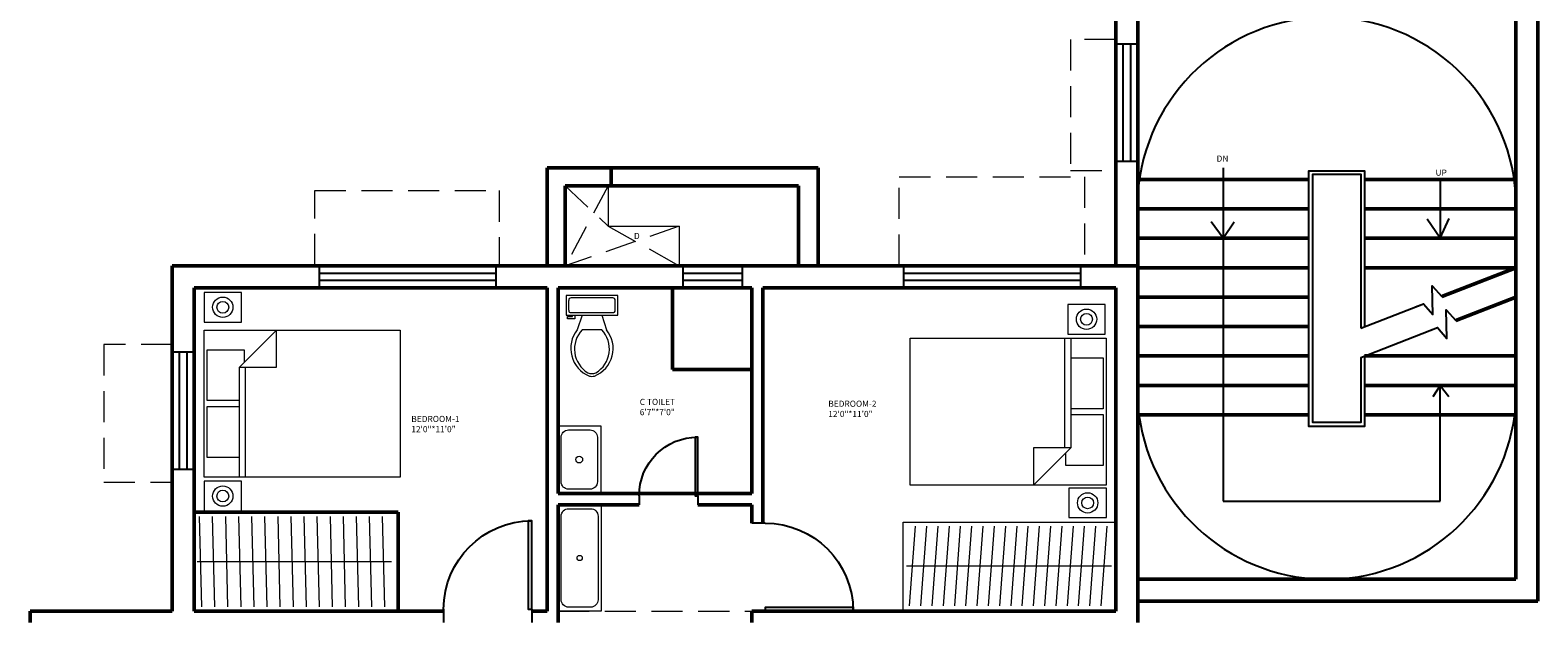
# Model space of a CAD drawing. Units: inches. Extents: x 4795 to 6024, y 2716 to 5025.
# Tile 11 of 19: x 4835 to 5450, y 4226 to 4465. Entities that reach past the tile are written whole.
import ezdxf

# ---------------------------------------------------------------- set-up
doc = ezdxf.new("R2010")
doc.units = ezdxf.units.IN
doc.linetypes.add('DASHED', pattern=[19.05, 12.7, -6.35])
for name, color, linetype, lineweight in [('A-ANNO-TEXT', 7, 'Continuous', 18), ('A-AREA-IDEN', 3, 'Continuous', 18), ('A-DOOR', 4, 'Continuous', 25), ('A-FLOR-FIXT', 9, 'Continuous', 18), ('A-FLOR-STRS', 3, 'Continuous', 25), ('A-FURN', 8, 'Continuous', 18), ('A-GLAZ', 4, 'Continuous', 25), ('A-WALL', 7, 'Continuous', 50), ('A-WALL-OVHD', 8, 'DASHED', 18)]:
    doc.layers.add(name, color=color, linetype=linetype, lineweight=lineweight)
doc.styles.get("Standard").update_dxf_attribs({"font": 'arial.ttf'})

# ---------------------------------------------------------------- blocks, each defined once
blk = doc.blocks.new('*U2')
for p, q in [((0, 0), (0, -6)), ((40, 0), (40, -6))]:
    blk.add_line(p, q)
blk.add_lwpolyline([(0, 0), (0, 40), (1.75, 40), (1.75, 0)], close=True)
blk.add_arc((0, 0), 40, 0, 90)
blk = doc.blocks.new('Bed - Queen')
for p, q in [((0, -80.00003), (0, 0)), ((0, 0), (59.99999, 0)), ((59.99999, 0), (59.99999, -80.00003)), ((7.99999, -1.2), (28.79998, -1.2)), ((7.99999, -14.4), (7.99999, -1.2)), ((28.79998, -1.2), (28.79998, -14.4)), ((31.19999, -1.2), (51.99999, -1.2)), ((31.19999, -14.4), (31.19999, -1.2)), ((51.99999, -1.2), (51.99999, -16.4)), ((0, -14.4), (44.8, -14.4)), ((44.8, -16.8), (0, -16.8)), ((59.99999, -29.6), (44.8, -14.4)), ((44.8, -14.4), (44.8, -29.6)), ((51.99999, -16.4), (46.79936, -16.4)), ((44.8, -29.6), (59.99999, -29.6)), ((59.99999, -80.00003), (0, -80.00003))]:
    blk.add_line(p, q)
blk = doc.blocks.new('Toilet - top')
for p, q in [((9.5, -6), (9.5, -2)), ((-10, -8.5), (-8, -8.5)), ((-10, -9.5), (-10, -8.5)), ((-7, -9.5), (-10, -9.5)), ((-8, -8.5), (-8, -8)), ((-7, -8), (-7, -9.5)), ((-4, -8), (-6, -14)), ((4, -8), (6, -14)), ((4, -14), (-4, -14))]:
    blk.add_line(p, q)
blk.add_lwpolyline([(10.5, -8), (10.5, 0), (-10.5, 0), (-10.5, -8)], close=True)
for points in [[(-9.5, -2), (-9.5, -6)], [(8.5, -1), (-8.5, -1)], [(-8.5, -7), (8.5, -7)]]:
    blk.add_lwpolyline(points)
for centre, radius, start, end in [((-8.62, -1.88), 0.884, 81.8699, 188.1301), ((-8.62, -6.12), 0.884, 171.8699, 278.1301), ((8.62, -1.88), 0.884, 351.8699, 98.1301), ((8.62, -6.12), 0.884, 261.8699, 8.1301), ((3.52, -21.58), 12.17, 141.46911, 247.97143), ((4.2, -21.82), 11.33, 136.36773, 238.94682), ((-3.52, -21.58), 12.17, 292.02843, 38.53071), ((-4.2, -21.82), 11.33, 301.05301, 43.63209), ((0, -27.88), 4, 245.73182, 294.26817), ((0, -29), 4, 254.86053, 285.13947)]:
    blk.add_arc(centre, radius, start, end)
blk = doc.blocks.new('WIN-48')
for p, q in [((0, 0), (0, 48)), ((0, 48), (9, 48)), ((3, 0), (3, 48)), ((6, 48), (6, 0)), ((9, 48), (9, 0)), ((9, 0), (0, 0))]:
    blk.add_line(p, q)
blk = doc.blocks.new('WIN-72')
for p, q in [((0, 0), (0, 9)), ((0, 9), (72, 9)), ((72, 9), (72, 0)), ((0, 6), (72, 6)), ((72, 3), (0, 3)), ((72, 0), (0, 0))]:
    blk.add_line(p, q)
blk = doc.blocks.new('WIN-24')
for p, q in [((0, 0), (0, 9)), ((0, 9), (24, 9)), ((24, 9), (24, 0)), ((0, 6), (24, 6)), ((24, 3), (0, 3)), ((24, 0), (0, 0))]:
    blk.add_line(p, q)

msp = doc.modelspace()

# ---------------------------------------------------------------- linework, layer by layer
at = {"layer": 'A-FLOR-FIXT'}
for points in [[(5050.47, 4275.81), (5068.01, 4275.81), (5068.01, 4303.28), (5050.47, 4303.28)], [(5050.47, 4271.31), (5067.98, 4271.31), (5067.98, 4227.81), (5050.47, 4227.81)]]:
    msp.add_lwpolyline(points, close=True, dxfattribs=at)
for points in [[(5054.67, 4301.8), (5063.47, 4301.8, -0.414214), (5066.47, 4298.8), (5066.47, 4280.62, -0.414214), (5063.47, 4277.62), (5054.67, 4277.62, -0.414214), (5051.67, 4280.62), (5051.67, 4298.8, -0.414214)], [(5054.69, 4269.65), (5063.78, 4269.65, -0.414214), (5066.78, 4266.65), (5066.78, 4232.51, -0.414214), (5063.78, 4229.51), (5054.69, 4229.51, -0.414214), (5051.69, 4232.51), (5051.69, 4266.65, -0.414214)]]:
    msp.add_lwpolyline(points, format="xyb", close=True, dxfattribs=at)
for centre, radius in [((5059.07, 4289.71), 1.38), ((5059.24, 4249.58), 1.06)]:
    msp.add_circle(centre, radius, dxfattribs=at)
at = {"layer": 'A-FLOR-STRS'}
for p, q in [((5321.88, 4408.72), (5321.88, 4272.68)), ((5410.38, 4403.98), (5410.38, 4379.98)), ((5321.88, 4379.98), (5316.99, 4386.66)), ((5321.88, 4379.98), (5326.34, 4386.66)), ((5410.38, 4379.98), (5405.1, 4387.75)), ((5410.38, 4379.98), (5414.06, 4388.08)), ((5378.02, 4343.39), (5403.52, 4353.31)), ((5378.02, 4331.39), (5409.28, 4343.55)), ((5410.38, 4319.98), (5407.44, 4315.34)), ((5410.38, 4272.68), (5410.38, 4319.98)), ((5410.38, 4319.98), (5413.85, 4315.44)), ((5321.88, 4272.68), (5410.38, 4272.68))]:
    msp.add_line(p, q, dxfattribs=at)
for points in [[(5379.55, 4331.98), (5379.55, 4303.18), (5356.8, 4303.18), (5356.8, 4407.51), (5379.55, 4407.51), (5379.55, 4343.98)], [(5378.02, 4331.39), (5378.02, 4304.79), (5358.4, 4304.79), (5358.4, 4406.15), (5378.02, 4406.15), (5378.02, 4343.39)], [(5400.24, 4352.03), (5403.52, 4353.31), (5407.38, 4348.91), (5407.12, 4360.6), (5410.98, 4356.21), (5414.26, 4357.49)], [(5406.45, 4342.45), (5409.28, 4343.55), (5413.14, 4339.15), (5412.88, 4350.85), (5416.74, 4346.45), (5419.56, 4347.55)]]:
    msp.add_lwpolyline(points, dxfattribs=at)
for centre, radius, start, end in [((5364.1, 4392.81), 77.28, 3.66327, 176.33673), ((5364.14, 4318.25), 77.36, 187.62852, 355.12022)]:
    msp.add_arc(centre, radius, start, end, dxfattribs=at)
at = {"layer": 'A-FURN'}
for p, q in [((5070.93, 4401.37), (5070.93, 4384.91)), ((5070.93, 4384.91), (5099.88, 4384.91)), ((5099.88, 4384.91), (5099.88, 4368.81)), ((4904, 4266.54), (4904.91, 4229.63)), ((4909.33, 4266.54), (4910.25, 4229.63)), ((4914.67, 4266.54), (4915.58, 4229.63)), ((4920.01, 4266.54), (4920.92, 4229.63)), ((4925.34, 4266.54), (4926.26, 4229.63)), ((4930.68, 4266.54), (4931.6, 4229.63)), ((4936.02, 4266.54), (4936.93, 4229.63)), ((4941.36, 4266.54), (4942.27, 4229.63)), ((4946.69, 4266.54), (4947.61, 4229.63)), ((4952.03, 4266.54), (4952.95, 4229.63)), ((4957.37, 4266.54), (4958.28, 4229.63)), ((4962.71, 4266.54), (4963.62, 4229.63)), ((4968.04, 4266.54), (4968.96, 4229.63)), ((4973.38, 4266.54), (4974.3, 4229.63)), ((4978.72, 4266.54), (4979.63, 4229.63)), ((5191.22, 4227.81), (5191.22, 4264.24)), ((5191.22, 4264.24), (5277.97, 4264.24)), ((5193.86, 4230.08), (5196.3, 4262.56)), ((5198.46, 4230.08), (5200.9, 4262.56)), ((5203.06, 4230.08), (5205.5, 4262.56)), ((5207.66, 4230.08), (5210.1, 4262.56)), ((5212.26, 4230.08), (5214.7, 4262.56)), ((5216.86, 4230.08), (5219.3, 4262.56)), ((5221.46, 4230.08), (5223.9, 4262.56)), ((5226.06, 4230.08), (5228.5, 4262.56)), ((5230.66, 4230.08), (5233.1, 4262.56)), ((5235.25, 4230.08), (5237.7, 4262.56)), ((5239.85, 4230.08), (5242.3, 4262.56)), ((5244.45, 4230.08), (5246.9, 4262.56)), ((5249.05, 4230.08), (5251.5, 4262.56)), ((5253.65, 4230.08), (5256.1, 4262.56)), ((5258.25, 4230.08), (5260.7, 4262.56)), ((5262.85, 4230.08), (5265.3, 4262.56)), ((5267.45, 4230.08), (5269.9, 4262.56)), ((5272.05, 4230.08), (5274.5, 4262.56)), ((4903.13, 4248.09), (4982.45, 4248.09)), ((5192.55, 4246.32), (5276.22, 4246.32))]:
    msp.add_line(p, q, dxfattribs=at)
for points in [[(4905.98, 4345.83), (4921.26, 4345.83), (4921.26, 4357.87), (4905.98, 4357.87)], [(5258.42, 4340.94), (5273.69, 4340.94), (5273.69, 4352.97), (5258.42, 4352.97)], [(4905.98, 4268.8), (4921.26, 4268.8), (4921.26, 4280.84), (4905.98, 4280.84)], [(5258.88, 4266.02), (5274.16, 4266.02), (5274.16, 4278.06), (5258.88, 4278.06)]]:
    msp.add_lwpolyline(points, close=True, dxfattribs=at)
for centre, radius in [((4913.62, 4351.85), 4.15), ((4913.62, 4351.85), 2.4), ((5266.06, 4346.95), 4.15), ((5266.06, 4346.95), 2.4), ((4913.62, 4274.82), 4.15), ((4913.62, 4274.82), 2.4), ((5266.52, 4272.04), 4.15), ((5266.52, 4272.04), 2.4)]:
    msp.add_circle(centre, radius, dxfattribs=at)
at = {"layer": 'A-WALL'}
for p, q in [((5277.97, 4507.98), (5277.97, 4368.81)), ((5286.97, 4507.98), (5286.97, 4223.31)), ((5441.22, 4470.09), (5441.22, 4240.93)), ((5450.22, 4470.09), (5450.22, 4231.93)), ((5045.97, 4408.73), (5156.53, 4408.73)), ((5045.97, 4408.73), (5045.97, 4368.81)), ((5072.1, 4408.73), (5072.1, 4401.37)), ((5156.53, 4408.73), (5156.53, 4368.81)), ((5053.37, 4368.81), (5053.37, 4401.37)), ((5053.37, 4401.37), (5148.57, 4401.37)), ((5148.57, 4401.37), (5148.57, 4368.81)), ((5286.97, 4403.98), (5356.8, 4403.98)), ((5379.55, 4403.98), (5441.22, 4403.98)), ((5286.97, 4391.98), (5356.8, 4391.98)), ((5379.55, 4391.98), (5441.22, 4391.98)), ((5286.97, 4379.98), (5356.8, 4379.98)), ((5379.55, 4379.98), (5441.22, 4379.98)), ((5286.97, 4368.81), (4892.97, 4368.81)), ((4892.97, 4368.81), (4892.97, 4227.81)), ((5286.97, 4367.98), (5356.8, 4367.98)), ((5379.55, 4367.98), (5441.22, 4367.98)), ((5410.98, 4356.21), (5441.22, 4367.98)), ((4901.97, 4359.81), (4901.97, 4227.81)), ((5045.97, 4359.81), (4901.97, 4359.81)), ((5045.97, 4359.81), (5045.97, 4227.81)), ((5050.47, 4359.81), (5050.47, 4275.81)), ((5129.47, 4359.81), (5050.47, 4359.81)), ((5097.17, 4359.81), (5097.17, 4326.44)), ((5129.47, 4359.81), (5129.47, 4275.81)), ((5277.97, 4359.81), (5133.97, 4359.81)), ((5133.97, 4359.81), (5133.97, 4263.81)), ((5277.97, 4359.81), (5277.97, 4227.81)), ((5286.97, 4355.98), (5356.8, 4355.98)), ((5416.74, 4346.45), (5441.22, 4355.98)), ((5286.97, 4343.98), (5356.8, 4343.98)), ((5286.97, 4331.98), (5356.8, 4331.98)), ((5379.55, 4331.98), (5441.22, 4331.98)), ((5097.17, 4326.44), (5129.47, 4326.44)), ((5286.97, 4319.98), (5356.8, 4319.98)), ((5379.55, 4319.98), (5441.22, 4319.98)), ((5286.97, 4307.98), (5356.8, 4307.98)), ((5379.55, 4307.98), (5441.22, 4307.98)), ((5129.47, 4275.81), (5050.47, 4275.81)), ((5050.47, 4271.31), (5050.47, 4223.31)), ((5083.47, 4271.31), (5050.47, 4271.31)), ((5129.47, 4271.31), (5107.47, 4271.31)), ((5129.47, 4271.31), (5129.47, 4263.81)), ((4901.97, 4268.24), (4985.17, 4268.24)), ((4985.17, 4268.24), (4985.17, 4227.81)), ((5441.22, 4240.93), (5286.97, 4240.93)), ((4892.97, 4227.81), (4835.02, 4227.81)), ((4835.02, 4227.81), (4835.02, 4223.31)), ((5003.74, 4227.81), (4901.97, 4227.81)), ((5045.97, 4227.81), (5039.74, 4227.81)), ((5277.97, 4227.81), (5129.47, 4227.81)), ((5129.47, 4227.81), (5129.47, 4223.31)), ((5450.22, 4231.93), (5286.97, 4231.93))]:
    msp.add_line(p, q, dxfattribs=at)
at = {"layer": 'A-WALL-OVHD'}
for p, q in [((5277.97, 4461.11), (5259.55, 4461.11)), ((5259.55, 4461.11), (5259.55, 4407.68)), ((5189.68, 4368.81), (5189.68, 4405.13)), ((5189.68, 4405.13), (5265.27, 4405.13)), ((5259.55, 4407.68), (5277.97, 4407.68)), ((5265.27, 4405.13), (5265.27, 4368.81)), ((4951.16, 4369.06), (4951.16, 4399.45)), ((4951.16, 4399.45), (5026.42, 4399.45)), ((5026.42, 4399.45), (5026.42, 4368.81)), ((5053.37, 4401.37), (5070.93, 4384.91)), ((5070.93, 4401.37), (5053.37, 4368.81)), ((5099.88, 4384.91), (5053.37, 4368.81)), ((5070.93, 4384.91), (5099.88, 4368.81)), ((4892.97, 4336.7), (4865.06, 4336.7)), ((4865.06, 4336.7), (4865.06, 4280.51)), ((4865.06, 4280.51), (4892.97, 4280.51)), ((5050.47, 4227.81), (5129.47, 4227.81))]:
    msp.add_line(p, q, dxfattribs=at)

# ---------------------------------------------------------------- block references
at = {"layer": 'A-DOOR'}
for p, xscale, yscale, zscale in [((5107.47, 4274.91), -0.6, 0.6, 0.6), ((5039.74, 4228.71), -0.9, 0.9, 0.9)]:
    msp.add_blockref('*U2', p, dxfattribs=dict(at, xscale=xscale, yscale=yscale, zscale=zscale))
at = {"layer": 'A-DOOR', "xscale": -0.9, "yscale": 0.9, "zscale": 0.9, "rotation": 270}
msp.add_blockref('*U2', (5134.87, 4227.81), dxfattribs=at)
at = {"layer": 'A-FLOR-FIXT'}
msp.add_blockref('Toilet - top', (5064.25, 4356.65), dxfattribs=at)
at = {"layer": 'A-FURN'}
for p, rotation in [((4905.98, 4282.55), 90), ((5274.04, 4339.24), 270)]:
    msp.add_blockref('Bed - Queen', p, dxfattribs=dict(at, rotation=rotation))
at = {"layer": 'A-GLAZ', "rotation": 180}
for name, p in [('WIN-48', (5286.97, 4459.28)), ('WIN-72', (5025.09, 4368.81)), ('WIN-24', (5125.54, 4368.81)), ('WIN-72', (5263.56, 4368.81)), ('WIN-48', (4901.97, 4333.7))]:
    msp.add_blockref(name, p, dxfattribs=at)

# ---------------------------------------------------------------- texts
at = {"layer": 'A-ANNO-TEXT', "char_height": 2.5, "attachment_point": 1}
for s, width, insert in [('DN', 10.2803, (5319.14, 4413.76)), ('UP', 5.3731, (5408.47, 4408.01)), ('D', 1.0897, (5081.4, 4382.19))]:
    msp.add_mtext_dynamic_manual_height_columns(s, width=width, gutter_width=12.5, heights=[0], dxfattribs=dict(at, insert=insert))
at = {"layer": 'A-AREA-IDEN', "char_height": 2.5, "attachment_point": 1}
for s, width, insert in [('C TOILET\\P6\'7"*7\'0"', 49.9824, (5083.76, 4314.49)), ('BEDROOM-2\\P12\'0"*11\'0"', 49.793, (5160.69, 4313.74)), ('BEDROOM-1\\P12\'0"*11\'0"', 50.564, (4990.55, 4307.54))]:
    msp.add_mtext_dynamic_manual_height_columns(s, width=width, gutter_width=12.5, heights=[0], dxfattribs=dict(at, insert=insert))

doc.saveas('drawing.dxf')
